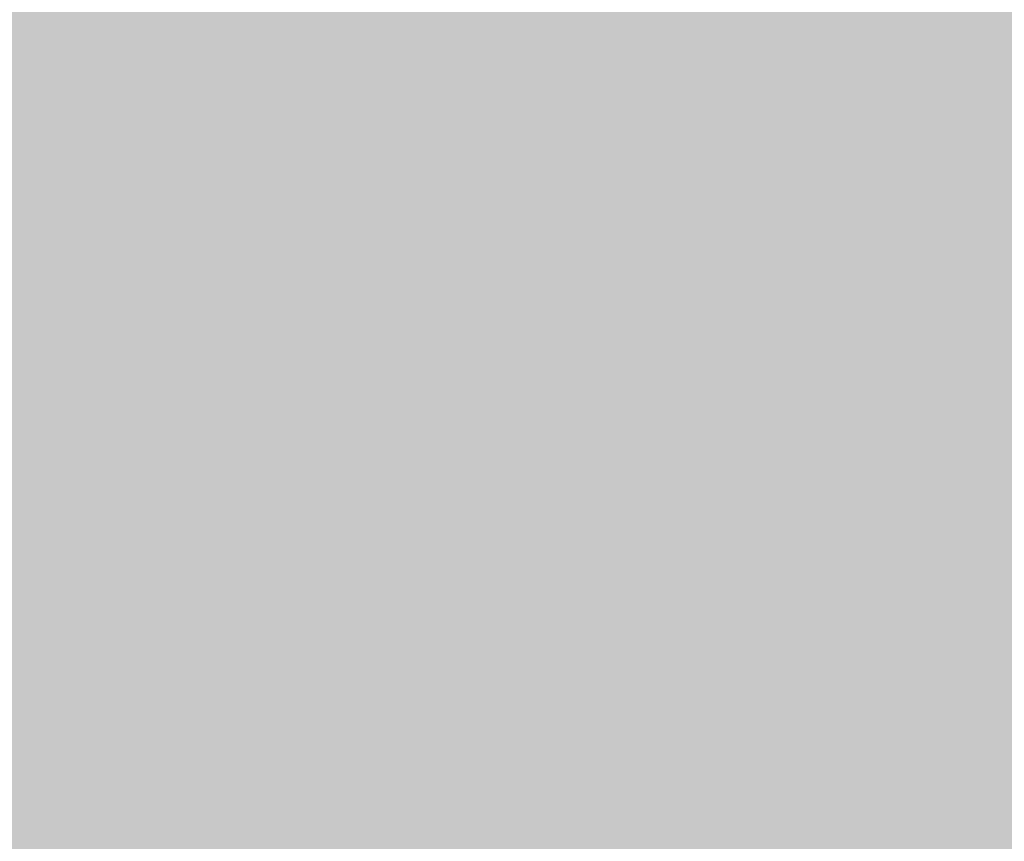
# Model space of a CAD drawing. Units: feet. Extents: x 3168 to 4724, y 827 to 1477.
# Tile 147 of 256: x 3301.14682 to 3301.1638, y 1099.00068 to 1099.01485. Entities that reach past the tile are written whole.
import ezdxf

# ---------------------------------------------------------------- set-up
doc = ezdxf.new("R2010")
doc.units = ezdxf.units.FT
doc.layers.add('A-ELEV', color=7, linetype='Continuous', lineweight=35)
doc.layers.add('A-ELEV-PATT', color=8, linetype='Continuous', lineweight=13)

msp = doc.modelspace()

# ---------------------------------------------------------------- hatches: boundary and pattern name
at = {"layer": 'A-ELEV-PATT'}
h = msp.add_hatch(color=256, dxfattribs=at)
h.dxf.hatch_style = 1
edge = h.paths.add_edge_path()
edge.add_ellipse((3552.905762, 979.220141), major_axis=(36.744924, 0), ratio=0.484848485, start_angle=0, end_angle=360)
edge = h.paths.add_edge_path()
edge.add_ellipse((3559.891637, 929.252282), major_axis=(36.744924, 0), ratio=0.484848485, start_angle=0, end_angle=360)
edge = h.paths.add_edge_path()
edge.add_line((3299.31681, 1198.606081), (3479.916714, 1198.606081))
edge.add_line((3479.916714, 1198.606081), (3479.916714, 1209.86857))
edge.add_spline(control_points=[(3479.916714, 1209.86857), (3464.301157, 1209.86857), (3448.685601, 1209.86857), (3410.949139, 1209.86857), (3388.828234, 1209.86857), (3355.646876, 1209.86857), (3344.586423, 1209.86857), (3327.995745, 1209.86857), (3322.465518, 1209.86857), (3314.170179, 1209.86857), (3311.405066, 1209.86857), (3307.257396, 1209.86857), (3305.874839, 1209.86857), (3303.801005, 1209.86857), (3303.109726, 1209.86857), (3302.072809, 1209.86857), (3301.72717, 1209.86857), (3301.208711, 1209.86857), (3301.035891, 1209.86857), (3300.776662, 1209.86857), (3300.690252, 1209.86857), (3300.560638, 1209.86857), (3300.517433, 1209.86857), (3300.452625, 1209.86857), (3300.431023, 1209.86857), (3300.398619, 1209.86857), (3300.387818, 1209.86857), (3300.366216, 1209.86857), (3300.345676, 1209.86857), (3300.345548, 1209.86857), (3300.345505, 1209.86857), (3300.343304, 1209.86857), (3300.341146, 1209.868571), (3300.337909, 1209.868571), (3300.33683, 1209.868572), (3300.333942, 1209.868573), (3300.332133, 1209.868574), (3300.325515, 1209.868577), (3300.320706, 1209.868581), (3300.310925, 1209.868592), (3300.305952, 1209.868598), (3300.290511, 1209.868623), (3300.280045, 1209.868646), (3300.232425, 1209.868777), (3300.195298, 1209.868954), (3299.951068, 1209.870608), (3299.744824, 1209.874326), (3299.436827, 1209.883257), (3299.334389, 1209.886792), (3299.181079, 1209.89292), (3299.130033, 1209.895099), (3298.652217, 1209.916801), (3298.22946, 1209.945718), (3297.601631, 1210.002367), (3297.393404, 1210.023464), (3297.082652, 1210.058309), (3296.979332, 1210.070458), (3296.292954, 1210.154861), (3295.718148, 1210.243356), (3294.868717, 1210.39885), (3294.5877, 1210.454478), (3294.169341, 1210.543349), (3294.030415, 1210.573878), (3291.707149, 1211.1012), (3289.65359, 1211.813435), (3285.776259, 1213.563988), (3283.95141, 1214.603478), (3280.512159, 1216.98008), (3278.897241, 1218.317592), (3276.379914, 1220.829489), (3275.416042, 1221.917738), (3274.039342, 1223.7077), (3273.581043, 1224.349535), (3273.143228, 1225.016316)], knot_values=[39.119033, 39.119033, 39.119033, 39.119033, 39.286353, 39.286353, 39.523379, 39.523379, 39.641892, 39.641892, 39.701148, 39.701148, 39.730777, 39.730777, 39.745591, 39.745591, 39.752998, 39.752998, 39.756701, 39.756701, 39.758553, 39.758553, 39.759479, 39.759479, 39.759942, 39.759942, 39.760173, 39.760173, 39.760289, 39.760289, 39.760405, 39.760405, 39.760463, 39.760463, 39.763389, 39.763389, 39.764851, 39.764851, 39.767304, 39.767304, 39.773825, 39.773825, 39.78057, 39.78057, 39.79477, 39.79477, 39.845194, 39.845194, 40.126715, 40.126715, 40.267476, 40.267476, 40.337856, 40.337856, 40.927023, 40.927023, 41.221606, 41.221606, 41.368898, 41.368898, 42.202622, 42.202622, 42.619485, 42.619485, 42.827916, 42.827916, 46.118323, 46.118323, 49.408731, 49.408731, 52.699139, 52.699139, 54.927489, 54.927489, 56.104228, 56.104228, 56.104228, 56.104228], weights=[1, 1, 1, 1, 1, 1, 1, 1, 1, 1, 1, 1, 1, 1, 1, 1, 1, 1, 1, 1, 1, 1, 1, 1, 1, 1, 1, 1, 1, 1, 1, 1, 1, 1, 1, 1, 1, 1, 1, 1, 1, 1, 1, 1, 1, 1, 1, 1, 1, 1, 1, 1, 1, 1, 1, 1, 1, 1, 1, 1, 1, 1, 1, 1, 1, 1, 1, 1, 1, 1, 1, 1, 1, 1], degree=3, periodic=0)
edge.add_line((3273.143228, 1225.016316), (3273.143228, 1099.016316))
edge.add_line((3273.143228, 1099.016316), (3299.31681, 1099.016316))
edge.add_line((3299.31681, 1099.016316), (3299.31681, 1198.606081))
edge = h.paths.add_edge_path()
edge.add_line((3304.758443, 1324.15806), (3479.916714, 1324.15806))
edge.add_line((3479.916714, 1324.15806), (3479.916714, 1335.714618))
edge.add_line((3479.916714, 1335.714618), (3269.161628, 1335.714618))
edge.add_spline(control_points=[(3269.161628, 1335.714618), (3264.024231, 1335.714618), (3258.364118, 1328.958189), (3259.264311, 1323.900274)], knot_values=[0, 0, 0, 0, 15.412191, 15.412191, 15.412191, 15.412191], degree=3, periodic=0)
edge.add_line((3259.264311, 1323.900274), (3265.516849, 1288.769135))
edge.add_line((3265.516849, 1288.769135), (3275.265103, 1261.545626))
edge.add_line((3275.265103, 1261.545626), (3304.758443, 1261.545626))
edge.add_line((3304.758443, 1261.545626), (3304.758443, 1324.15806))
h = msp.add_hatch(color=256, dxfattribs=at)
h.dxf.hatch_style = 1
h.paths.add_polyline_path([(3384.525247, 1099.016316), (3335.029168, 1099.016316), (3299.31681, 1099.016316), (3273.143228, 1099.016316), (3217.565364, 1099.016316), (3168.069285, 827.11626), (3335.029168, 827.11626)])

# ---------------------------------------------------------------- linework, layer by layer
at = {"layer": 'A-ELEV'}
msp.add_open_spline([(3808.5202, 1099.016316), (3808.5202, 1141.413235), (3808.5202, 1183.810154), (3808.5202, 1226.635324), (3808.5202, 1227.063576), (3808.5202, 1227.491828), (3811.491871, 1248.994673), (3814.463542, 1270.497518), (3817.46523, 1292.217564), (3817.495247, 1292.434764), (3817.525264, 1292.651964), (3817.572801, 1310.106748), (3817.620339, 1327.561532), (3817.667877, 1345.016316), (3817.667877, 1345.457962), (3817.667877, 1345.899608), (3817.667877, 1346.456047), (3817.667877, 1346.57084), (3817.667877, 1346.752887), (3817.667877, 1346.820142), (3817.667877, 1346.93487), (3817.667877, 1346.982345), (3817.667877, 1347.038587), (3817.667877, 1347.047356), (3817.667877, 1347.073661), (3817.667877, 1347.059303), (3817.667877, 1347.061545), (3817.667876, 1347.062667), (3817.667875, 1347.066031), (3817.667874, 1347.068274), (3817.66787, 1347.075001), (3817.667866, 1347.079486), (3817.667849, 1347.092937), (3817.667833, 1347.101902), (3817.667766, 1347.12879), (3817.667699, 1347.146705), (3817.667432, 1347.200421), (3817.667165, 1347.236192), (3817.6661, 1347.343385), (3817.665038, 1347.414686), (3817.660812, 1347.628095), (3817.656608, 1347.769708), (3817.63997, 1348.192487), (3817.623509, 1348.471586), (3817.559094, 1349.300067), (3817.496121, 1349.840588), (3817.255432, 1351.424156), (3817.026318, 1352.428785), (3816.306871, 1354.888914), (3815.743745, 1356.268727), (3814.463959, 1358.81921), (3813.746413, 1359.990968), (3812.195838, 1362.172343), (3811.362245, 1363.182124), (3809.588836, 1365.069009), (3808.648816, 1365.946105), (3806.654262, 1367.579616), (3805.599702, 1368.336154), (3803.352891, 1369.722327), (3802.160535, 1370.352386), (3799.600813, 1371.453586), (3798.232688, 1371.925481), (3795.280084, 1372.634624), (3793.693148, 1372.872068), (3791.869441, 1372.92648), (3791.740861, 1372.92922), (3791.353371, 1372.934101), (3791.092707, 1372.932901), (3790.304116, 1372.915068), (3789.769543, 1372.884195), (3789.20919, 1372.830236), (3789.190622, 1372.828424), (3789.134892, 1372.822912), (3789.097705, 1372.819137), (3789.048445, 1372.814008), (3789.0364, 1372.812743), (3789.000256, 1372.808918), (3788.976147, 1372.806325), (3788.949405, 1372.803404), (3788.946786, 1372.803118), (3788.942567, 1372.802655), (3788.940967, 1372.80248), (3788.938572, 1372.802217), (3788.937777, 1372.802129), (3788.935391, 1372.801867), (3788.867535, 1372.794402), (3788.756866, 1372.782228), (3788.701532, 1372.776141), (3788.53553, 1372.75788), (3788.424861, 1372.745707), (3788.092856, 1372.709185), (3787.871519, 1372.684837), (3787.207509, 1372.611793), (3786.764835, 1372.563097), (3785.436814, 1372.417009), (3784.551467, 1372.319617), (3781.895425, 1372.027442), (3780.12473, 1371.832658), (3774.812646, 1371.248307), (3771.271256, 1370.858739), (3760.647088, 1369.690037), (3753.56431, 1368.910902), (3732.315973, 1366.573498), (3718.150416, 1365.015228), (3694.006758, 1362.359326), (3684.028657, 1361.261694), (3674.050557, 1360.164062), (3664.600662, 1360.164062), (3655.150767, 1360.164062), (3626.801081, 1360.164062), (3607.901291, 1360.164062), (3551.20192, 1360.164062), (3513.40234, 1360.164062), (3467.725182, 1360.164062), (3459.847604, 1360.164062), (3436.214873, 1360.164062), (3420.459718, 1360.164062), (3373.194255, 1360.164062), (3341.683946, 1360.164062), (3302.848162, 1360.164062), (3295.522686, 1360.164062), (3286.038292, 1360.164062), (3283.879372, 1360.164062), (3277.402613, 1360.164062), (3273.084773, 1360.164062), (3267.732851, 1360.164062), (3266.698768, 1360.164062), (3263.59652, 1360.164062), (3261.528355, 1360.164062), (3259.236943, 1360.164062), (3259.013697, 1360.164062), (3258.343958, 1360.164062), (3257.897466, 1360.164062), (3257.430998, 1360.164062), (3257.411022, 1360.164062), (3257.370573, 1360.164062), (3257.37547, 1360.164062), (3257.374598, 1360.164062), (3257.373937, 1360.164062), (3257.371956, 1360.164062), (3257.370635, 1360.164061), (3257.366673, 1360.16406), (3257.364032, 1360.164059), (3257.356109, 1360.164053), (3257.350828, 1360.164047), (3257.334987, 1360.164023), (3257.32443, 1360.163998), (3257.292769, 1360.163899), (3257.271676, 1360.163799), (3257.208439, 1360.163398), (3257.166337, 1360.162995), (3257.040206, 1360.161388), (3256.956349, 1360.159783), (3256.705504, 1360.153393), (3256.53924, 1360.147036), (3256.04357, 1360.121916), (3255.717296, 1360.097102), (3254.752446, 1360.000481), (3254.127968, 1359.906513), (3252.180067, 1359.525332), (3250.941574, 1359.143991), (3248.670175, 1358.24329), (3247.635739, 1357.723834), (3245.732632, 1356.603471), (3244.863388, 1356.00206), (3243.253108, 1354.742865), (3242.511972, 1354.084731), (3240.751052, 1352.344781), (3239.800961, 1351.229574), (3238.087769, 1348.87244), (3237.324685, 1347.630355), (3235.98251, 1344.971632), (3235.402205, 1343.554907), (3234.591081, 1340.815458), (3234.310882, 1339.54355), (3233.97649, 1336.802561), (3233.922113, 1335.330877), (3234.148916, 1332.591269), (3234.349529, 1331.367201), (3234.719893, 1329.999367), (3234.752423, 1329.883362), (3234.853619, 1329.534797), (3234.925892, 1329.301685), (3235.024836, 1329.002552), (3235.046924, 1328.936928), (3235.077639, 1328.847239), (3235.085924, 1328.823198), (3235.110939, 1328.751064), (3235.127828, 1328.702962), (3235.147992, 1328.646242), (3235.151059, 1328.637632), (3235.156096, 1328.623526), (3235.158061, 1328.61803), (3235.160209, 1328.61203), (3235.165612, 1328.596943), (3235.180099, 1328.556486), (3235.190263, 1328.528101), (3235.220756, 1328.442946), (3235.241084, 1328.386176), (3235.302069, 1328.215865), (3235.342726, 1328.102325), (3235.464696, 1327.761704), (3235.54601, 1327.534623), (3235.78995, 1326.853381), (3235.952577, 1326.39922), (3236.440459, 1325.036736), (3236.765713, 1324.128414), (3237.741475, 1321.403446), (3238.391983, 1319.586801), (3240.343508, 1314.136866), (3241.644525, 1310.503576), (3245.547574, 1299.603706), (3248.149607, 1292.337126), (3255.955706, 1270.537385), (3261.159772, 1256.004225), (3267.387618, 1238.612001), (3268.411397, 1235.752937), (3269.510378, 1232.683864), (3269.585579, 1232.473854), (3269.706612, 1232.135851), (3269.752444, 1232.007857), (3269.827329, 1231.79873), (3269.856382, 1231.717595), (3269.906325, 1231.578122), (3269.927215, 1231.519782), (3269.972468, 1231.393406), (3269.996831, 1231.325368), (3270.026503, 1231.242506), (3270.031811, 1231.227681), (3270.040282, 1231.204024), (3270.039224, 1231.206979), (3270.039359, 1231.206601), (3270.039427, 1231.206412), (3270.03963, 1231.205846), (3270.039765, 1231.205468), (3270.040171, 1231.204335), (3270.040442, 1231.203579), (3270.041254, 1231.201313), (3270.041796, 1231.199802), (3270.04342, 1231.195269), (3270.044504, 1231.192248), (3270.047756, 1231.183185), (3270.049926, 1231.177145), (3270.056442, 1231.159028), (3270.060793, 1231.146957), (3270.073867, 1231.110761), (3270.082613, 1231.086656), (3270.108936, 1231.014413), (3270.1266, 1230.96635), (3270.179934, 1230.822457), (3270.215947, 1230.726923), (3270.325323, 1230.441508), (3270.400026, 1230.252811), (3270.629249, 1229.691444), (3270.788883, 1229.323501), (3271.286488, 1228.238319), (3271.6431, 1227.539755), (3272.775859, 1225.515277), (3273.614169, 1224.260502), (3275.416042, 1221.917738), (3276.379914, 1220.829489), (3278.897241, 1218.317592), (3280.512159, 1216.98008), (3283.95141, 1214.603478), (3285.776259, 1213.563988), (3289.65359, 1211.813435), (3291.707149, 1211.1012), (3294.030415, 1210.573878), (3294.169341, 1210.543349), (3294.5877, 1210.454478), (3294.868717, 1210.39885), (3295.718148, 1210.243356), (3296.292954, 1210.154861), (3296.979332, 1210.070458), (3297.082652, 1210.058309), (3297.393404, 1210.023464), (3297.601631, 1210.002367), (3298.22946, 1209.945718), (3298.652217, 1209.916801), (3299.130033, 1209.895099), (3299.181079, 1209.89292), (3299.334389, 1209.886792), (3299.436827, 1209.883257), (3299.744824, 1209.874326), (3299.951068, 1209.870608), (3300.195298, 1209.868954), (3300.232425, 1209.868777), (3300.280045, 1209.868646), (3300.290511, 1209.868623), (3300.305952, 1209.868598), (3300.310925, 1209.868592), (3300.320706, 1209.868581), (3300.325515, 1209.868577), (3300.332133, 1209.868574), (3300.333942, 1209.868573), (3300.33683, 1209.868572), (3300.337909, 1209.868571), (3300.341146, 1209.868571), (3300.343304, 1209.86857), (3300.345505, 1209.86857), (3300.345548, 1209.86857), (3300.345676, 1209.86857), (3300.366216, 1209.86857), (3300.387818, 1209.86857), (3300.398619, 1209.86857), (3300.431023, 1209.86857), (3300.452625, 1209.86857), (3300.517433, 1209.86857), (3300.560638, 1209.86857), (3300.690252, 1209.86857), (3300.776662, 1209.86857), (3301.035891, 1209.86857), (3301.208711, 1209.86857), (3301.72717, 1209.86857), (3302.072809, 1209.86857), (3303.109726, 1209.86857), (3303.801005, 1209.86857), (3305.874839, 1209.86857), (3307.257396, 1209.86857), (3311.405066, 1209.86857), (3314.170179, 1209.86857), (3322.465518, 1209.86857), (3327.995745, 1209.86857), (3344.586423, 1209.86857), (3355.646876, 1209.86857), (3388.828234, 1209.86857), (3410.949139, 1209.86857), (3477.311855, 1209.86857), (3521.553665, 1209.86857), (3566.836184, 1209.86857), (3567.876892, 1209.86857), (3570.999017, 1209.86857), (3573.080433, 1209.86857), (3575.781396, 1209.86857), (3576.400943, 1209.86857), (3577.295821, 1209.86857), (3577.571152, 1209.86857), (3578.397146, 1209.86857), (3578.947808, 1209.86857), (3579.756491, 1209.86857), (3580.014511, 1209.86857), (3580.342737, 1209.86857), (3580.326865, 1209.86857), (3580.32717, 1209.86857), (3580.327323, 1209.86857), (3580.327781, 1209.86857), (3580.328086, 1209.86857), (3580.329002, 1209.86857), (3580.329613, 1209.86857), (3580.331445, 1209.86857), (3580.332667, 1209.86857), (3580.336332, 1209.868569), (3580.338775, 1209.868567), (3580.346107, 1209.868563), (3580.350995, 1209.868558), (3580.365663, 1209.86854), (3580.375445, 1209.868522), (3580.404801, 1209.868449), (3580.424386, 1209.868376), (3580.483183, 1209.868085), (3580.522437, 1209.867793), (3580.640361, 1209.866624), (3580.719195, 1209.865454), (3580.956315, 1209.860766), (3581.115222, 1209.85607), (3581.594164, 1209.83723), (3581.916419, 1209.818331), (3582.889947, 1209.742428), (3583.547986, 1209.666169), (3585.531827, 1209.360617), (3586.867216, 1209.053886), (3589.471545, 1208.252472), (3590.740241, 1207.757852), (3591.995451, 1207.158802), (3592.057809, 1207.12874), (3592.244242, 1207.037954), (3592.367676, 1206.976632), (3592.73528, 1206.790359), (3592.976752, 1206.663101), (3593.244539, 1206.516441), (3593.274731, 1206.499825), (3593.365115, 1206.449839), (3593.425113, 1206.416333), (3593.604314, 1206.315285), (3593.722725, 1206.247211), (3593.857212, 1206.168398), (3593.874362, 1206.158319), (3593.925741, 1206.128041), (3593.959899, 1206.107798), (3594.062086, 1206.046899), (3594.129827, 1206.006074), (3594.208436, 1205.958171), (3594.219683, 1205.951304), (3594.253391, 1205.930686), (3594.275819, 1205.916917), (3594.342972, 1205.875536), (3594.387563, 1205.847853), (3594.433616, 1205.81905), (3594.435256, 1205.818024), (3594.440175, 1205.814946), (3594.443453, 1205.812894), (3594.447123, 1205.810594), (3594.447516, 1205.810348), (3594.448695, 1205.80961), (3594.449481, 1205.809117), (3594.450366, 1205.808562), (3594.450466, 1205.8085), (3594.4506, 1205.808415), (3594.467399, 1205.797887), (3594.493269, 1205.781674), (3594.506204, 1205.773568), (3594.545008, 1205.749248), (3594.570878, 1205.733035), (3594.648487, 1205.684396), (3594.700226, 1205.651969), (3594.855444, 1205.554691), (3594.958922, 1205.489839), (3595.269357, 1205.295282), (3595.476314, 1205.165577), (3596.097185, 1204.776463), (3596.511099, 1204.517054), (3597.752841, 1203.738826), (3598.580669, 1203.220007), (3601.064152, 1201.663551), (3602.719807, 1200.625914), (3607.686774, 1197.513002), (3610.998085, 1195.437727), (3620.932018, 1189.211903), (3627.55464, 1185.061354), (3647.422507, 1172.609707), (3660.667751, 1164.308608), (3700.403484, 1139.405313), (3726.893973, 1122.803116), (3757.205715, 1103.806052), (3761.02697, 1101.411184), (3764.848224, 1099.016316), (3745.328271, 1099.016316), (3725.808319, 1099.016316), (3706.288366, 1099.016316), (3706.288366, 1108.453237), (3706.288366, 1117.890158), (3706.288366, 1127.327079), (3710.750754, 1127.327079), (3715.213143, 1127.327079), (3719.675531, 1127.327079)], degree=3, knots=[0, 0, 0, 0, 0.982037, 0.982037, 0.991957, 0.991957, 0.991957, 1.966522, 1.966522, 1.976367, 1.976367, 1.976367, 2.976367, 2.976367, 2.976367, 3.00169, 3.00169, 3.008272, 3.008272, 3.012129, 3.012129, 3.014851, 3.014851, 3.015353, 3.015353, 3.016359, 3.016359, 3.017365, 3.017365, 3.019376, 3.019376, 3.023398, 3.023398, 3.031442, 3.031442, 3.047531, 3.047531, 3.079708, 3.079708, 3.144063, 3.144063, 3.272772, 3.272772, 3.53019, 3.53019, 4.045026, 4.045026, 5.074698, 5.074698, 6.700878, 6.700878, 8.327058, 8.327058, 9.953238, 9.953238, 11.579418, 11.579418, 13.205598, 13.205598, 14.831778, 14.831778, 16.457958, 16.457958, 18.084138, 18.084138, 18.206872, 18.206872, 18.45234, 18.45234, 18.943275, 18.943275, 18.960093, 18.960093, 18.993729, 18.993729, 19.00461, 19.00461, 19.026374, 19.026374, 19.028737, 19.028737, 19.03018, 19.03018, 19.030897, 19.030897, 19.032332, 19.032332, 19.033766, 19.033766, 19.036636, 19.036636, 19.042374, 19.042374, 19.053851, 19.053851, 19.076805, 19.076805, 19.122714, 19.122714, 19.21453, 19.21453, 19.398163, 19.398163, 19.765429, 19.765429, 20.024128, 20.024128, 20.024128, 20.092031, 20.092031, 20.227836, 20.227836, 20.499446, 20.499446, 20.556051, 20.556051, 20.66926, 20.66926, 20.895678, 20.895678, 20.948316, 20.948316, 20.963829, 20.963829, 20.994855, 20.994855, 21.002285, 21.002285, 21.017146, 21.017146, 21.01875, 21.01875, 21.021959, 21.021959, 21.022102, 21.022102, 21.022249, 21.022249, 21.022708, 21.022708, 21.023627, 21.023627, 21.025464, 21.025464, 21.029138, 21.029138, 21.036486, 21.036486, 21.051183, 21.051183, 21.080575, 21.080575, 21.139361, 21.139361, 21.256932, 21.256932, 21.492073, 21.492073, 21.962356, 21.962356, 23.01002, 23.01002, 24.057684, 24.057684, 25.105348, 25.105348, 26.153011, 26.153011, 27.776787, 27.776787, 29.400562, 29.400562, 31.024337, 31.024337, 32.278801, 32.278801, 33.533265, 33.533265, 34.467568, 34.467568, 34.553971, 34.553971, 34.726776, 34.726776, 34.775309, 34.775309, 34.793079, 34.793079, 34.82862, 34.82862, 34.834979, 34.834979, 34.839039, 34.839039, 34.839411, 34.839411, 34.840285, 34.840285, 34.842034, 34.842034, 34.845531, 34.845531, 34.852525, 34.852525, 34.866512, 34.866512, 34.894488, 34.894488, 34.950439, 34.950439, 35.062342, 35.062342, 35.286147, 35.286147, 35.733758, 35.733758, 35.821815, 35.821815, 35.828283, 35.828283, 35.832225, 35.832225, 35.834724, 35.834724, 35.836521, 35.836521, 35.838617, 35.838617, 35.839073, 35.839073, 35.839345, 35.839345, 35.839617, 35.839617, 35.840161, 35.840161, 35.841249, 35.841249, 35.843425, 35.843425, 35.847778, 35.847778, 35.856482, 35.856482, 35.873891, 35.873891, 35.908709, 35.908709, 35.978345, 35.978345, 36.117617, 36.117617, 36.396161, 36.396161, 36.953248, 36.953248, 38.067423, 38.067423, 40.295772, 40.295772, 42.524122, 42.524122, 45.81453, 45.81453, 49.104937, 49.104937, 52.395345, 52.395345, 52.603776, 52.603776, 53.020639, 53.020639, 53.854363, 53.854363, 54.001655, 54.001655, 54.296238, 54.296238, 54.885405, 54.885405, 54.955785, 54.955785, 55.096546, 55.096546, 55.378067, 55.378067, 55.42849, 55.42849, 55.442691, 55.442691, 55.449436, 55.449436, 55.455957, 55.455957, 55.458409, 55.458409, 55.459872, 55.459872, 55.462798, 55.462798, 55.462856, 55.462856, 55.462972, 55.462972, 55.463088, 55.463088, 55.463319, 55.463319, 55.463782, 55.463782, 55.464708, 55.464708, 55.46656, 55.46656, 55.470263, 55.470263, 55.47767, 55.47767, 55.492484, 55.492484, 55.522112, 55.522112, 55.581369, 55.581369, 55.699882, 55.699882, 55.936907, 55.936907, 56.410959, 56.410959, 56.42211, 56.42211, 56.444413, 56.444413, 56.451051, 56.451051, 56.454001, 56.454001, 56.459901, 56.459901, 56.462666, 56.462666, 56.463418, 56.463418, 56.464171, 56.464171, 56.465675, 56.465675, 56.468684, 56.468684, 56.474702, 56.474702, 56.486738, 56.486738, 56.51081, 56.51081, 56.558955, 56.558955, 56.655243, 56.655243, 56.847821, 56.847821, 57.232975, 57.232975, 58.003284, 58.003284, 59.543901, 59.543901, 62.625137, 62.625137, 68.787607, 68.787607, 74.950078, 74.950078, 75.27336, 75.27336, 75.919923, 75.919923, 77.213051, 77.213051, 77.377769, 77.377769, 77.707206, 77.707206, 78.366079, 78.366079, 78.462532, 78.462532, 78.655436, 78.655436, 79.041245, 79.041245, 79.105735, 79.105735, 79.234714, 79.234714, 79.492672, 79.492672, 79.502197, 79.502197, 79.521249, 79.521249, 79.523534, 79.523534, 79.528103, 79.528103, 79.528682, 79.528682, 79.528885, 79.528885, 79.529089, 79.529089, 79.529495, 79.529495, 79.530308, 79.530308, 79.531935, 79.531935, 79.535187, 79.535187, 79.541693, 79.541693, 79.554704, 79.554704, 79.580725, 79.580725, 79.632769, 79.632769, 79.736856, 79.736856, 79.94503, 79.94503, 80.361377, 80.361377, 80.421435, 80.421435, 80.421435, 81.421435, 81.421435, 81.421435, 82.421435, 82.421435, 82.421435, 83.421435, 83.421435, 83.421435, 83.421435], dxfattribs=at)

doc.saveas('drawing.dxf')
